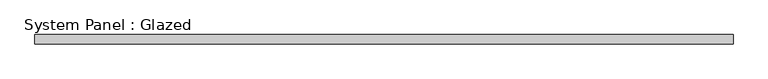
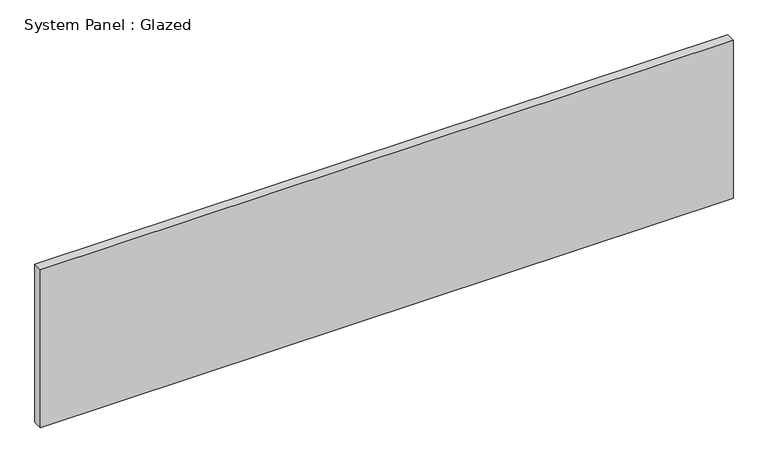
"""IFC4 building model written with IfcOpenShell, lengths in millimetres: plate geometry, System Panel : Glazed."""

from ifc_helpers import new_model, si_unit, origin, origin_with_axes, place, context, project, spatial, polyline, outline, extrude, source, transform, mapped, element, save


def system_panel_glazed_7d5859e6(model_context):
    return source(origin(), model_context, "Body", "SweptSolid", [
        extrude(outline(polyline([(950.7907705, 19.05), (-950.7907705, 19.05), (-950.7907705, 44.45), (950.7907705, 44.45), (950.7907705, 19.05)])), origin_with_axes(), (0.0, 0.0, 1.0), 458.4735266),
    ])


if __name__ == "__main__":
    model = new_model("IFC4")
    model_context = context("Model", 3, world=origin())
    ifc_project = project(units=[si_unit("LENGTHUNIT", "METRE", prefix="MILLI")], contexts=[model_context])
    site = spatial("IfcSite", under=ifc_project)
    building = spatial("IfcBuilding", under=site)
    placement = place(None, origin())
    system_panel_glazed_shape = system_panel_glazed_7d5859e6(model_context)
    element("IfcPlate", 1, ObjectType="System Panel : Glazed", at=placement, inside=building, context=model_context, shape_type="MappedRepresentation", body=[
        mapped(system_panel_glazed_shape, transform((0.0, 0.0, 0.0), x_axis=(1.0, 0.0, 0.0), y_axis=(0.0, 1.0, 0.0), z_axis=(0.0, 0.0, 1.0))),
    ])
    save(model, "model.ifc")

# Revit data of these elements
# Type "System Panel : Glazed"
#   Construction Type Id = "GSP4R"
#   Analytic Construction = "1/8 in Pilkington single glazing"
#   Visual Light Transmittance = 0.9
#   Solar Heat Gain Coefficient = 0.86
#   Heat Transfer Coefficient (U) = 1.18115 BTU/(h·ft²·°F)
#   Define Thermal Properties by = 1
# Element 1 (IfcPlate, "System Panel : Glazed")
#   Materials on its faces: "Glass"
# Materials
#   "Glass": class "Glass", colour RGB 0 128 192, transparency 0.75, Description = "Soda Lime Glass", Cost = 0
